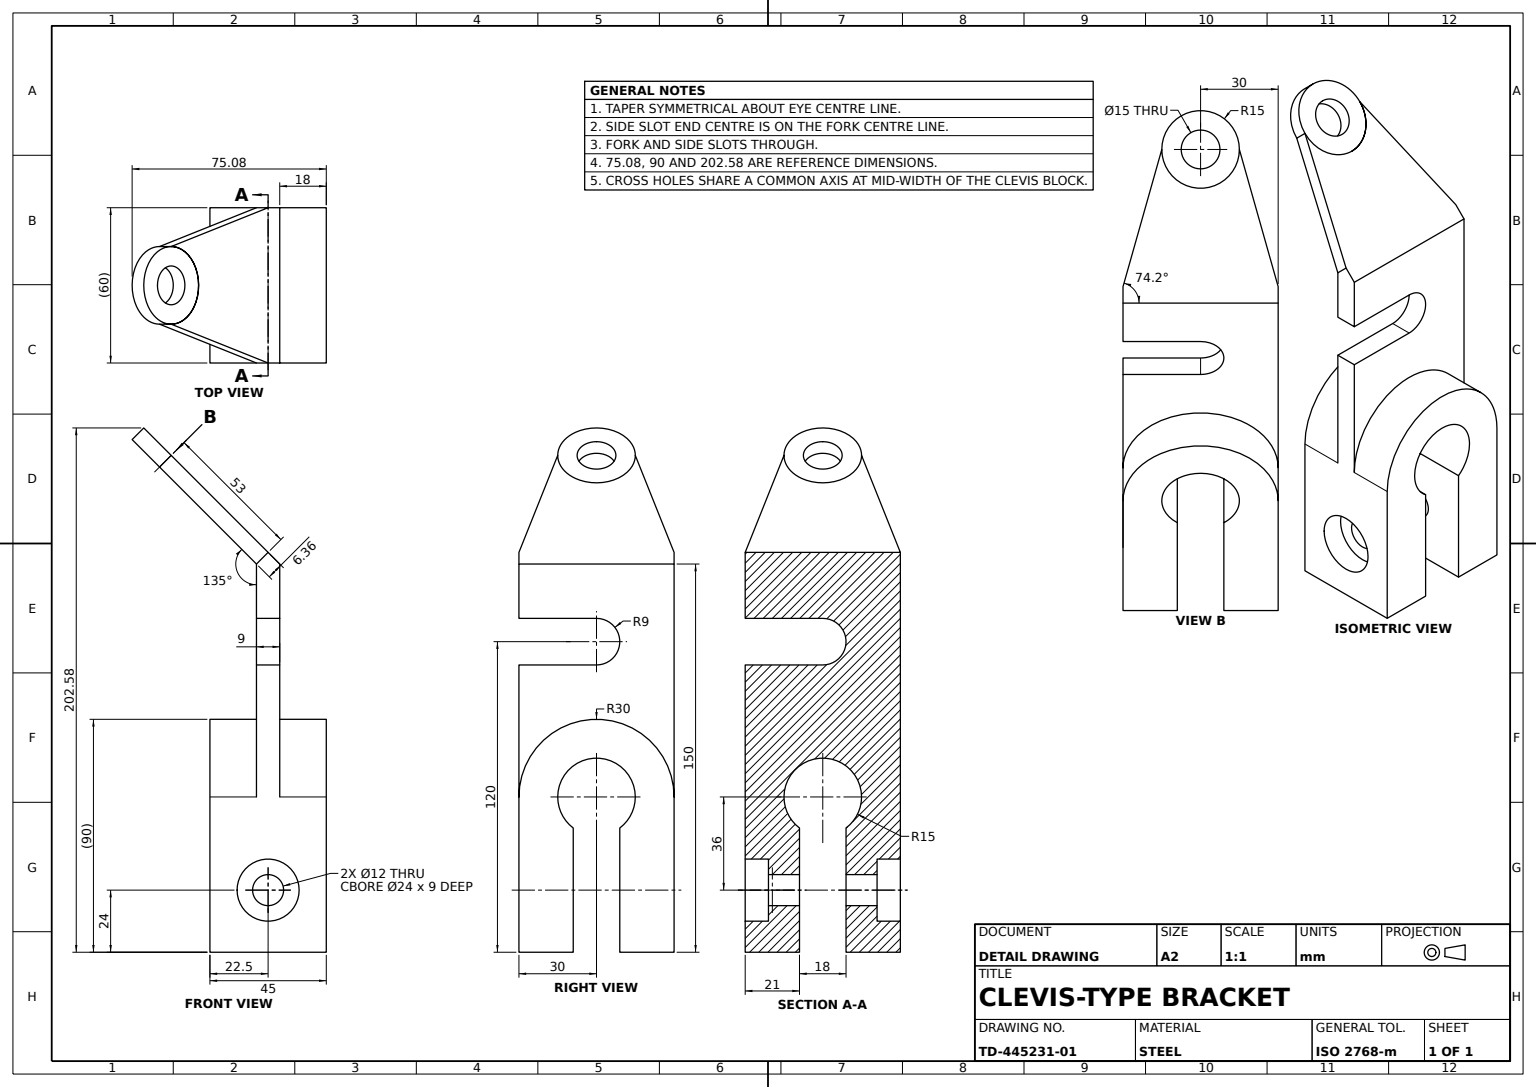
SolidWorks part; units mm, degrees
material "Plain Carbon Steel"
ref_plane "Front Plane" through (0, 0, 0) normal (0, 0, 1) x (1, 0, 0)
ref_plane "Top Plane" through (0, 0, 0) normal (0, 1, 0) x (1, 0, 0)
ref_plane "Right Plane" through (0, 0, 0) normal (1, 0, 0) x (0, 0, -1)
sketch "Clevis Block Profile" plane through (0, 0, 0) normal (0, 0, 1) x (1, 0, 0)
  line L0 (0, 0) -> (30, 0)
  line L1 (30, 0) -> (30, 60)
  line L3 (-30, 60) -> (-30, 0)
  line L4 (-30, 0) -> (0, 0)
  arc A0 (30, 60) -> (-30, 60) centre (0, 60) ccw
  point P7 (0, 90)
  dimension "D1" = 30
  dimension "D4" = 60
  dimension "D2" = 90
  dimension "D3" = 60
extrude "Clevis Block" add sketch "Clevis Block Profile" along normal mid plane 45
sketch "Fork Slot Profile" plane through (0, 0, 22.5) normal (0, 0, 1) x (1, 0, 0)
  line L0 (0, 0) -> (9, 0)
  line L1 (-30, 0) -> (30, 0) construction
  line L2 (9, 0) -> (9, 48)
  line L3 (-9, 0) -> (0, 0)
  line L4 (-9, 48) -> (-9, 0)
  line L5 (30, 0) -> (30, 60) construction
  arc A0 (9, 48) -> (-9, 48) centre (0, 60) ccw
  dimension "D1" = 15
  dimension "D2" = 21
extrude "Fork Slot" cut sketch "Fork Slot Profile" against normal blind 64
sketch "Side Hole A Profile" plane through (-30, 0, 0) normal (-1, 0, 0) x (0, 0, 1)
  line L0 (-22.5, 60) -> (-22.5, 0) construction
  line L1 (22.5, 0) -> (-22.5, 0) construction
  circle A0 centre (0, 24) radius 12
  dimension "D1" = 24
  dimension "D2" = 22.5
  dimension "D3" = 24
extrude "Side Hole A" cut sketch "Side Hole A Profile" against normal blind 9
sketch "Side Hole B Profile" plane through (30, 0, 0) normal (1, 0, 0) x (0, 0, -1)
  line L0 (22.5, 0) -> (22.5, 60) construction
  line L1 (-22.5, 60) -> (22.5, 60) construction
  circle A0 centre (0, 24) radius 12
  dimension "D1" = 24
  dimension "D2" = 22.5
  dimension "D3" = 36
extrude "Side Hole B" cut sketch "Side Hole B Profile" against normal blind 9
sketch "Cross Hole Profile" plane through (21, 0, 0) normal (1, 0, 0) x (0, 0, -1)
  circle A0 centre (0, 24) radius 6
  dimension "D1" = 12
extrude "Cross Hole" cut sketch "Cross Hole Profile" against normal blind 51
sketch "Arm Plate Profile" plane through (0, 0, 0) normal (0, 0, 1) x (1, 0, 0)
  line L0 (-30, 60) -> (-30, 150)
  line L1 (-30, 150) -> (30, 150)
  line L2 (30, 150) -> (30, 60)
  arc A0 (30, 60) -> (-30, 60) centre (0, 60) ccw
  dimension "D1" = 150
extrude "Arm Plate" add sketch "Arm Plate Profile" along normal mid plane 9
ref_plane "Plane2" through (30, 0, 0) normal (1, 0, 0) x (0, 0, -1)
sketch "Bracket Web Profile" plane through (30, 0, 0) normal (1, 0, 0) x (0, 0, -1)
  line L0 (4.5, 150) -> (-32.9767, 187.4767)
  line L1 (-4.5, 150) -> (-41.9767, 187.4767)
  line L2 (-41.9767, 187.4767) -> (-37.4767, 191.9767)
  line L3 (-32.9767, 187.4767) -> (-37.4767, 191.9767)
  line L4 (-4.5, 150) -> (4.5, 150)
  dimension "D1" = 37.4767
extrude "Bracket Web" add sketch "Bracket Web Profile" against normal blind 60
sketch "Pin Boss Profile" plane through (0, 72.75, -72.75) normal (0, -0.7071, 0.7071) x (1, 0, 0)
  line L0 (-30, 162.248) -> (30, 162.248) construction
  circle A0 centre (0, 162.248) radius 15
  dimension "D1" = 30
extrude "Pin Boss" add sketch "Pin Boss Profile" against normal blind 9
sketch "Hook Slot Profile" plane through (0, 72.75, -72.75) normal (0, -0.7071, 0.7071) x (1, 0, 0)
  line L0 (-15, 162.248) -> (-30, 109.248)
  line L1 (-30, 109.248) -> (-30, 162.248)
  line L2 (-30, 162.248) -> (-15, 162.248)
  line L3 (15, 162.248) -> (30, 109.248)
  line L4 (30, 109.248) -> (30, 162.248)
  line L5 (30, 162.248) -> (15, 162.248)
extrude "Hook Slot" cut sketch "Hook Slot Profile" against normal blind 9
sketch "Boss Recess Profile" plane through (0, 79.114, -79.114) normal (0, 0.7071, -0.7071) x (1, 0, 0)
  circle A0 centre (0, -162.248) radius 15
  dimension "D1" = 30
extrude "Boss Recess 2mm" cut sketch "Boss Recess Profile" against normal blind 2
sketch "Boss Bore Profile" plane through (0, 77.6997, -77.6997) normal (0, 0.7071, -0.7071) x (1, 0, 0)
  circle A0 centre (0, -162.248) radius 15
  dimension "D1" = 30
extrude "Boss Bore" cut sketch "Boss Bore Profile" against normal blind 16
sketch "Bore Insert Boss Profile" plane through (0, 72.75, -72.75) normal (0, -0.7071, 0.7071) x (1, 0, 0)
  circle A0 centre (0, 162.248) radius 15
  dimension "D1" = 30
extrude "Bore Insert Boss" add sketch "Bore Insert Boss Profile" against normal blind 6.36
sketch "Insert Bore Profile" plane through (0, 72.75, -72.75) normal (0, -0.7071, 0.7071) x (1, 0, 0)
  circle A0 centre (0, 162.248) radius 7.5
  dimension "D1" = 15
extrude "Insert Bore" cut sketch "Insert Bore Profile" against normal blind 26.36
sketch "Arm Trim Profile" plane through (0, 0, 4.5) normal (0, 0, 1) x (1, 0, 0)
  line L0 (30, 60) -> (30, 120)
  line L1 (30, 60) -> (30, 150) construction
  line L3 (0, 129) -> (30, 129)
  line L4 (0, 111) -> (30, 111)
  line L5 (30, 111) -> (30, 129)
  arc A0 (0, 129) -> (0, 111) centre (0, 120) ccw
  line M6 (30, 60) -> (30, 150)
  dimension "D1" = 9
  dimension "D2" = 30
  dimension "D3" = 60
extrude "Arm Trim Cut" cut sketch "Arm Trim Profile" against normal blind 26.36 contours L3 A0 L4 L0 M6
